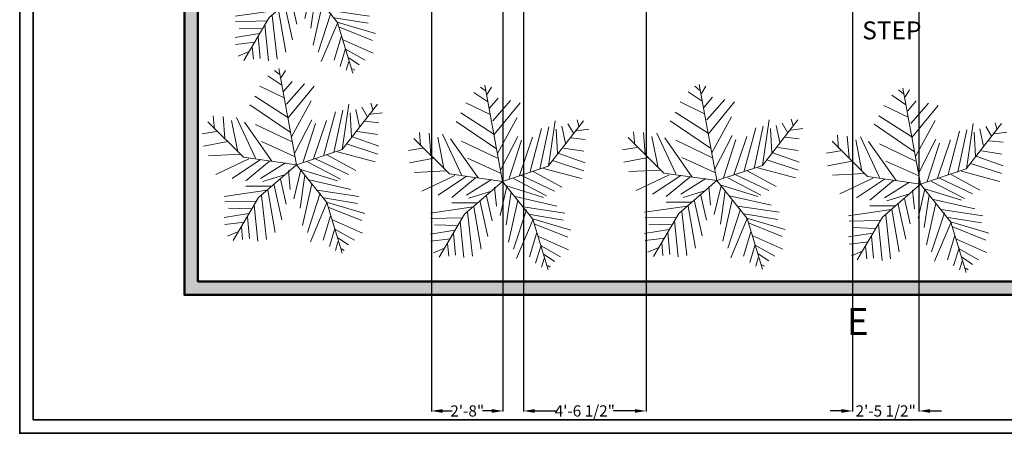
# Model space of a CAD drawing. Units: inches. Extents: x -60 to 743, y -483 to 510.
# Tile 1 of 7: x -60 to 378, y -483 to -299. Entities that reach past the tile are written whole.
import ezdxf

# ---------------------------------------------------------------- set-up
doc = ezdxf.new("R2010")
doc.units = ezdxf.units.IN
doc.header["$MEASUREMENT"] = 0
for name, color, linetype, lineweight in [('A-ANNO-DIMS', 2, 'Continuous', 18), ('A-ANNO-SYMB', 7, 'Continuous', 18), ('A-ANNO-TEXT', 7, 'Continuous', 25), ('A-ANNO-TTLB', 7, 'Continuous', 35), ('A-WALL-PATT', 30, 'Continuous', 13), ('TREES', 80, 'Continuous', 13), ('WALL BOUNDRY', 10, 'Continuous', 50)]:
    doc.layers.add(name, color=color, linetype=linetype, lineweight=lineweight)
doc.styles.get("Standard").update_dxf_attribs({"font": 'arial.ttf'})
doc.dimstyles.get("Standard").update_dxf_attribs({"dimtxt": 5, "dimasz": 5, "dimexe": 0.18, "dimexo": 0.0625, "dimgap": 0.09, "dimtad": 0, "dimtih": 1, "dimtoh": 1, "dimdec": 1, "dimzin": 0, "dimdsep": 46, "dimlunit": 4, "dimtxsty": 'Standard', "dimcen": 0.09, "dimadec": 0, "dimazin": 0, "dimtfac": 1, "dimtdec": 1, "dimtofl": 0, "dimtmove": 0, "dimatfit": 3, "dimfxl": 1, "dimtolj": 1, "dimtzin": 0, "dimarcsym": 0})

# ---------------------------------------------------------------- blocks, each defined once
blk = doc.blocks.new('*U21')
for p, q in [((-221.9198, 1197.3052), (-433.5526, 1338.8594)), ((-258.7244, 1362.456), (-332.3336, 1421.4348)), ((0, 0), (-266.7, 1447.8)), ((-231.1146, 1315.2628), (-166.7002, 1421.4348)), ((-194.31, 1102.9442), (-65.4812, 1256.284)), ((-148.3106, 914.1968), (118.5418, 1220.9018)), ((-185.1152, 1008.5578), (-553.1612, 1185.4942)), ((-129.8956, 701.8528), (265.7602, 1185.4942)), ((-93.091, 489.5342), (-700.3796, 902.3858)), ((-129.8956, 713.6638), (-626.7704, 1032.1544)), ((-74.7014, 418.7444), (219.7608, 961.39)), ((685.8, 228.6), (1219.2, 914.4)), ((689.0258, 230.0224), (790.2448, 914.1968)), ((1121.4862, 925.9824), (1149.0706, 831.6214)), ((412.9786, 147.447), (587.8068, 796.2392)), ((560.197, 182.8292), (698.2206, 819.8358)), ((808.6344, 784.4282), (827.0494, 418.7444)), ((891.4384, 831.6214), (946.658, 572.1096)), ((983.4626, 867.0036), (1066.2666, 725.4494)), ((1112.2914, 760.8316), (1296.3144, 784.4282)), ((-800.1, 114.3), (-1333.5, 647.7)), ((-1234.059, 536.7274), (-1252.4486, 737.2604)), ((-1105.2302, 725.4494), (-1077.6458, 395.1732)), ((-976.4268, 666.4706), (-884.4026, 194.6402)), ((-902.8176, 713.6638), (-617.5756, 100.2538)), ((-369.1382, 53.086), (-783.1836, 642.874)), ((-617.5756, 607.4918), (-74.7014, 347.98)), ((-28.6766, 171.0436), (228.9556, 678.2816)), ((100.1268, 41.275), (284.1498, 619.2774)), ((256.5654, 88.4682), (449.7832, 666.4706)), ((1029.462, 654.685), (1241.0948, 631.0884)), ((-1206.4492, 501.3198), (-1418.082, 465.9376)), ((919.0482, 501.3198), (1222.6798, 454.152)), ((-1031.621, 347.98), (-1399.667, 277.1902)), ((-525.5514, 347.98), (-28.6766, 123.8504)), ((753.4148, 312.5978), (1222.6798, 159.2326)), ((845.439, 418.7444), (1241.0948, 277.1902)), ((-847.598, 159.2326), (-1326.0578, 135.636)), ((0, 0), (685.8, 228.6)), ((615.4166, 194.6402), (1185.8752, 41.275)), ((-718.7946, 88.4682), (-1215.644, -147.447)), ((-543.9664, 76.6572), (-967.2066, -206.4512)), ((0, 0), (-800.1, 114.3)), ((-405.9428, 53.086), (-764.794, -241.8334)), ((0, 0), (-571.5, -495.3)), ((-166.7002, 29.4894), (-543.9664, -206.4512)), ((0, 0), (457.2, -571.5)), ((164.5412, 41.275), (661.416, -218.2368)), ((284.1498, 88.4682), (781.0246, -147.447)), ((458.978, 147.447), (891.4384, -88.4682)), ((-166.7002, -147.447), (-507.1618, -253.619)), ((-120.7008, -88.4682), (-93.091, -371.5766)), ((63.3222, -76.6826), (-37.8714, -513.1308)), ((44.9326, -64.897), (615.4166, -241.8334)), ((-341.5284, -289.0012), (-221.9198, -831.6214)), ((-240.3094, -218.2368), (-157.5054, -595.7062)), ((127.7366, -159.258), (54.1274, -654.685)), ((228.9556, -289.0012), (90.932, -914.1968)), ((192.151, -230.0224), (817.8292, -371.5766)), ((-442.7474, -383.3876), (-1086.8406, -477.7486)), ((-387.5278, -324.4088), (-764.794, -324.4088)), ((-433.5526, -383.3876), (-323.1134, -1020.3688)), ((357.759, -430.5554), (164.5412, -1020.3688)), ((311.7596, -383.3876), (937.4378, -477.7486)), ((-617.5756, -548.5384), (-1077.6458, -560.324)), ((-571.5, -495.3), (-952.5, -1143)), ((-525.5514, -465.963), (-451.9422, -1126.5408)), ((458.978, -572.1096), (210.5406, -1161.923)), ((412.9786, -501.3452), (919.0482, -583.9206)), ((457.2, -571.5), (685.8, -1333.5)), ((468.1982, -572.1096), (1029.462, -737.2604)), ((-718.7946, -737.2604), (-1086.8406, -796.2392)), ((-681.9646, -666.496), (-1022.4262, -654.685)), ((-635.9652, -607.5172), (-580.771, -1150.1374)), ((486.5878, -642.8994), (983.4626, -843.4324)), ((-783.1836, -867.029), (-1077.6458, -902.4112)), ((-737.1842, -784.4536), (-709.5744, -1114.7298)), ((514.1976, -772.6426), (403.7838, -1138.3264)), ((541.8074, -831.6214), (992.6574, -1032.1544)), ((-875.2078, -1008.5832), (-1040.8412, -1079.3476)), ((-829.2084, -937.7934), (-810.7934, -1126.5408)), ((578.612, -961.39), (495.7826, -1232.7128)), ((578.612, -973.1756), (873.0488, -1138.3264)), ((624.6114, -1161.923), (587.8068, -1291.6916)), ((624.6114, -1102.9442), (781.0246, -1209.1162)), ((679.8056, -1268.095), (716.6102, -1291.6916))]:
    blk.add_line(p, q)
blk = doc.blocks.new('*D69')
at = {"layer": 'A-ANNO-DIMS', "color": 0, "lineweight": -2, "transparency": 16777216}
for p, q in [((310.62, 340.16), (310.62, -473.51)), ((340.15, 340.16), (340.15, -473.51)), ((305.62, -473.33), (300.62, -473.33)), ((345.15, -473.33), (350.15, -473.33))]:
    blk.add_line(p, q, dxfattribs=at)
at = {"layer": 'A-ANNO-DIMS', "color": 0, "transparency": 16777216}
for points in [[(305.62, -472.5), (305.62, -474.17), (310.62, -473.33)], [(345.15, -472.5), (345.15, -474.17), (340.15, -473.33)]]:
    blk.add_solid(points, dxfattribs=at)
at = {"layer": 'Defpoints', "color": 0, "transparency": 16777216}
for p in [(310.62, 340.23), (340.15, 340.23), (340.15, -473.33)]:
    blk.add_point(p, dxfattribs=at)
at = {"layer": 'A-ANNO-DIMS', "color": 0, "transparency": 16777216, "insert": (325.38, -473.33), "char_height": 5, "attachment_point": 5}
blk.add_mtext('\\A1;2\'-5 1/2"', dxfattribs=at)
blk = doc.blocks.new('*D76')
at = {"layer": 'A-ANNO-DIMS', "color": 0, "lineweight": -2, "transparency": 16777216}
for p, q in [((154.99, -224.11), (154.99, -473.51)), ((123.15, -256.64), (123.15, -473.51)), ((128.15, -473.33), (132.29, -473.33)), ((149.99, -473.33), (145.85, -473.33))]:
    blk.add_line(p, q, dxfattribs=at)
at = {"layer": 'A-ANNO-DIMS', "color": 0, "transparency": 16777216}
for points in [[(128.15, -472.5), (128.15, -474.17), (123.15, -473.33)], [(149.99, -472.5), (149.99, -474.17), (154.99, -473.33)]]:
    blk.add_solid(points, dxfattribs=at)
at = {"layer": 'Defpoints', "color": 0, "transparency": 16777216}
for p in [(154.99, -224.05), (123.15, -256.58), (154.99, -473.33)]:
    blk.add_point(p, dxfattribs=at)
at = {"layer": 'A-ANNO-DIMS', "color": 0, "transparency": 16777216, "insert": (139.07, -473.33), "char_height": 5, "attachment_point": 5}
blk.add_mtext('\\A1;2\'-8"', dxfattribs=at)
blk = doc.blocks.new('*D79')
at = {"layer": 'A-ANNO-DIMS', "color": 0, "lineweight": -2, "transparency": 16777216}
for p, q in [((164.13, -262.18), (164.13, -473.51)), ((218.7, -262.64), (218.7, -473.51)), ((169.13, -473.33), (178.75, -473.33)), ((213.7, -473.33), (204.07, -473.33))]:
    blk.add_line(p, q, dxfattribs=at)
at = {"layer": 'A-ANNO-DIMS', "color": 0, "transparency": 16777216}
for points in [[(169.13, -472.5), (169.13, -474.17), (164.13, -473.33)], [(213.7, -472.5), (213.7, -474.17), (218.7, -473.33)]]:
    blk.add_solid(points, dxfattribs=at)
at = {"layer": 'Defpoints', "color": 0, "transparency": 16777216}
for p in [(164.13, -262.12), (218.7, -262.58), (218.7, -473.33)]:
    blk.add_point(p, dxfattribs=at)
at = {"layer": 'A-ANNO-DIMS', "color": 0, "transparency": 16777216, "insert": (191.41, -473.33), "char_height": 5, "attachment_point": 5}
blk.add_mtext('\\A1;4\'-6 1/2"', dxfattribs=at)

msp = doc.modelspace()

# ---------------------------------------------------------------- hatches: boundary and pattern name
at = {"layer": 'A-WALL-PATT'}
h = msp.add_hatch(color=256, dxfattribs=at)
h.dxf.hatch_style = 1
h.paths.add_polyline_path([(412.35, 168.77), (415.89, 168.77), (415.89, 114.92), (412.35, 114.92)], flags=16)
h.paths.add_polyline_path([(87.81, -138.81), (87.81, -142.35), (48.31, -142.32), (48.31, -138.78)], flags=16)
h.paths.add_polyline_path([(459.53, -138.78), (513.39, -138.78), (513.39, -142.32), (459.53, -142.32)], flags=16)
h.paths.add_polyline_path([(164.84, -257.78), (218.7, -257.78), (218.7, -261.32), (164.84, -261.32)], flags=16)
h.paths.add_polyline_path([(417.15, 114.92), (415.89, 114.92), (415.89, 168.77), (417.15, 168.77), (417.15, 195.42), (411.15, 195.42), (411.15, 168.77), (412.35, 168.77), (412.35, 114.92), (411.15, 114.92), (411.15, 28.42), (610.15, 28.42), (610.15, -43.58), (508.15, -43.58), (508.15, -49.58), (610.15, -49.58), (610.15, -137.58), (513.39, -137.58), (513.39, -138.78), (459.53, -138.78), (459.53, -137.58), (359.15, -137.58), (359.15, -143.58), (377.15, -143.58), (377.15, -292.58), (383.15, -292.58), (383.15, -143.58), (459.53, -143.58), (459.53, -142.32), (513.39, -142.32), (513.39, -143.58), (610.15, -143.58), (610.15, -415.58), (610.15, -421.58), (616.15, -421.58), (616.15, 418.42), (13.15, 418.42), (13.15, -421.58), (19.15, -421.58), (430.15, -421.58), (430.15, -415.58), (19.15, -415.58), (19.15, -143.58), (48.31, -143.58), (48.31, -142.32), (87.81, -142.35), (87.81, -143.58), (117.15, -143.58), (117.15, -262.58), (164.84, -262.58), (164.84, -261.32), (218.7, -261.32), (218.7, -262.58), (273.15, -262.58), (273.15, -292.58), (279.15, -292.58), (279.15, -143.58), (297.15, -143.58), (297.15, -137.58), (273.15, -137.58), (273.15, -256.58), (218.7, -256.58), (218.7, -257.78), (164.84, -257.78), (164.84, -256.58), (123.15, -256.58), (123.15, -143.58), (225.15, -143.58), (225.15, -137.58), (87.81, -137.58), (87.81, -138.81), (48.31, -138.78), (48.31, -137.58), (19.15, -137.58), (19.15, 28.42), (187.15, 28.42), (187.15, 34.42), (19.15, 34.42), (19.15, 178.42), (273.15, 178.42), (273.15, 184.42), (19.15, 184.42), (19.15, 345.58), (195.14, 345.58), (195.14, 348.9), (19.15, 348.9), (19.15, 412.42), (267.15, 412.42), (267.15, 319.83), (273.15, 319.83), (273.15, 412.42), (411.15, 412.42), (411.15, 376.24), (417.15, 376.24), (417.15, 412.42), (610.15, 412.42), (610.15, 249.42), (411.15, 249.42), (411.15, 243.42), (610.15, 243.42), (610.15, 34.42), (417.15, 34.42)])

# ---------------------------------------------------------------- linework, layer by layer
at = {"layer": 'A-ANNO-TTLB'}
for points in [[(742.84, -483.31), (-60.19, -483.31), (-60.19, 510.12), (742.84, 510.12)], [(736.84, -477.31), (-54.19, -477.31), (-54.19, 504.12), (736.84, 504.12)]]:
    msp.add_lwpolyline(points, close=True, dxfattribs=at)
at = {"layer": 'WALL BOUNDRY'}
msp.add_lwpolyline([(610.15, -415.58), (610.15, -421.58), (616.15, -421.58), (616.15, 418.42), (13.15, 418.42), (13.15, -421.58), (19.15, -421.58), (430.15, -421.58), (430.15, -415.58), (19.15, -415.58), (19.15, -143.58), (117.15, -143.58), (117.15, -262.58), (273.15, -262.58), (273.15, -292.58), (279.15, -292.58), (377.15, -292.58), (383.15, -292.58), (383.15, -143.58), (610.15, -143.58)], close=True, dxfattribs=at)

# ---------------------------------------------------------------- block references
at = {"layer": 'TREES', "xscale": 0.0295751403229488, "yscale": 0.0295751403229488, "zscale": 0.0295751403229488}
for p in [(67.83, -283.26), (63.05, -363.56), (154.8, -370.98), (250.19, -370.65), (340.92, -372.23)]:
    msp.add_blockref('*U21', p, dxfattribs=at)

# ---------------------------------------------------------------- texts
at = {"layer": 'A-ANNO-SYMB'}
msp.add_text('E', height=12, dxfattribs=at).set_placement((308.09, -439.45))
at = {"layer": 'A-ANNO-TEXT'}
msp.add_text('STEP', height=8, dxfattribs=at).set_placement((314.93, -307.68))

# ---------------------------------------------------------------- dimensions: what is measured, and where the dimension line sits
at = {"layer": 'A-ANNO-DIMS'}
for base, p1, p2, picture, middle in [((340.15, -473.33), (310.62, 340.23), (340.15, 340.23), '*D69', (325.38, -473.33)), ((154.99, -473.33), (123.15, -256.58), (154.99, -224.05), '*D76', (139.07, -473.33)), ((218.7, -473.33), (164.13, -262.12), (218.7, -262.58), '*D79', (191.41, -473.33))]:
    dim = msp.add_linear_dim(base=base, p1=p1, p2=p2, dimstyle='Standard', override={"dimdec": 1, "dimlfac": 1, "dimrnd": 0, "dimzin": 1, "dimdsep": 46, "dimlunit": 4, "dimfrac": 2}, dxfattribs=at)
    dim.commit()
    dim.dimension.update_dxf_attribs({"geometry": picture, "text_midpoint": middle})

doc.saveas('drawing.dxf')
